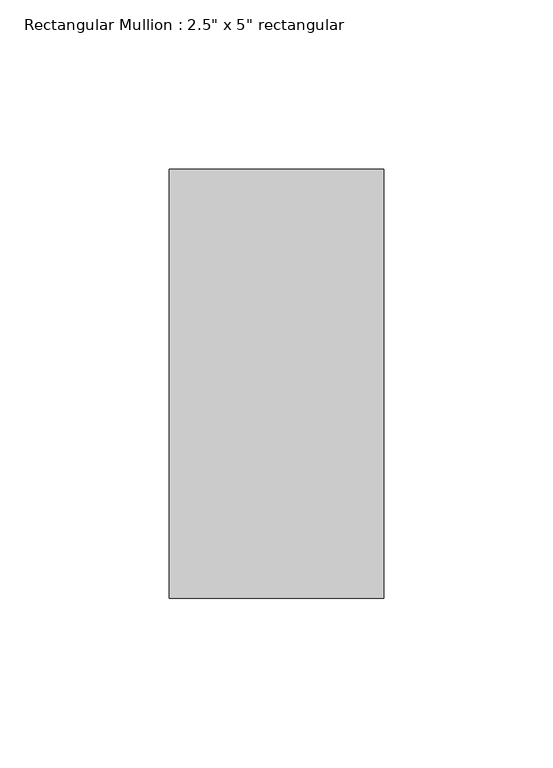
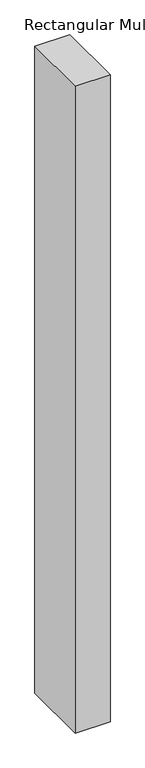
"""IFC4 building model written with IfcOpenShell, lengths in millimetres: member geometry."""

from ifc_helpers import new_model, si_unit, frame, origin, place, context, project, spatial, polyline, outline, extrude, source, transform, mapped, element, save


def member_a1da5be3(model_context):
    return source(origin(), model_context, "Body", "SweptSolid", [
        extrude(outline(polyline([(31.75, 63.5), (31.75, -63.5), (-31.75, -63.5), (-31.75, 63.5), (31.75, 63.5)])), frame((0.0, 0.0, -1244.6), z_axis=(0.0, 0.0, 1.0), x_axis=(1.0, 0.0, 0.0)), (0.0, 0.0, 1.0), 1244.6),
    ])


if __name__ == "__main__":
    model = new_model("IFC4")
    model_context = context("Model", 3, world=origin())
    ifc_project = project(units=[si_unit("LENGTHUNIT", "METRE", prefix="MILLI")], contexts=[model_context])
    site = spatial("IfcSite", under=ifc_project)
    building = spatial("IfcBuilding", under=site)
    placement = place(None, origin())
    member_shape = member_a1da5be3(model_context)
    element("IfcMember", 1, ObjectType="Rectangular Mullion : 2.5\" x 5\" rectangular", at=placement, inside=building, context=model_context, shape_type="MappedRepresentation", body=[
        mapped(member_shape, transform((0.0, 0.0, 0.0), x_axis=(1.0, 0.0, 0.0), y_axis=(0.0, 1.0, 0.0), z_axis=(0.0, 0.0, 1.0))),
    ])
    save(model, "model.ifc")

# Revit data of these elements
# Type "Rectangular Mullion : 2.5\" x 5\" rectangular"
#   built-in parameter 1007304 = 0.416667 (stored number, unit not read)
#   built-in parameter 1007301 = 0.104167 (stored number, unit not read)
#   built-in parameter 1007300 = 0.104167 (stored number, unit not read)
